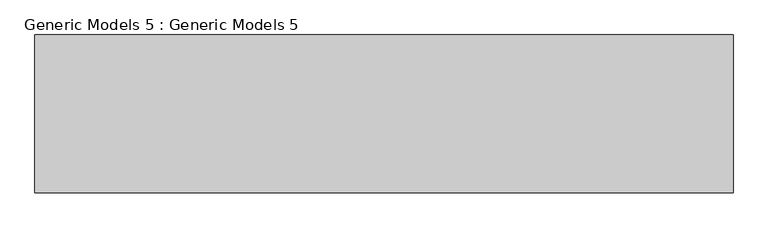
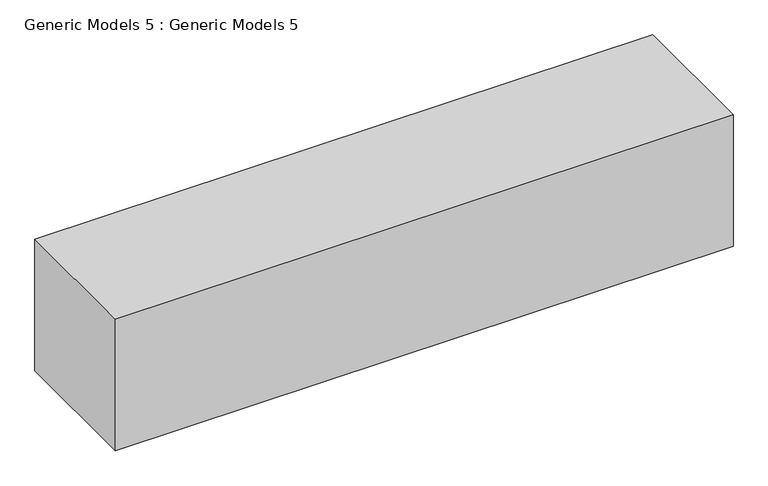
"""IFC4 building model written with IfcOpenShell, lengths in millimetres: proxy geometry, Generic Models 5 : Generic Models 5."""

from ifc_helpers import new_model, si_unit, frame, origin, place, context, project, spatial, polyline, outline, extrude, source, transform, mapped, element, save


def generic_models_5_generic_models_5_ea9a58cb(model_context):
    return source(origin(), model_context, "Body", "SweptSolid", [
        extrude(outline(polyline([(5025.7248685, -14083.1167162), (5025.7248685, -14845.1167162), (1652.8739931, -14845.1167162), (1652.8739931, -14083.1167162), (5025.7248685, -14083.1167162)])), frame((0.0, 0.0, 5799.1653852), z_axis=(0.0, 0.0, 1.0), x_axis=(1.0, 0.0, 0.0)), (0.0, 0.0, 1.0), 757.3100336),
    ])


if __name__ == "__main__":
    model = new_model("IFC4")
    model_context = context("Model", 3, world=origin())
    ifc_project = project(units=[si_unit("LENGTHUNIT", "METRE", prefix="MILLI")], contexts=[model_context])
    site = spatial("IfcSite", under=ifc_project)
    building = spatial("IfcBuilding", under=site)
    placement = place(None, origin())
    generic_models_5_generic_models_5_shape = generic_models_5_generic_models_5_ea9a58cb(model_context)
    element("IfcBuildingElementProxy", 1, Name="Generic Models 5 : Generic Models 5", ObjectType="Generic Models 5 : Generic Models 5", at=placement, inside=building, context=model_context, shape_type="MappedRepresentation", body=[
        mapped(generic_models_5_generic_models_5_shape, transform((0.0, 0.0, 0.0), x_axis=(1.0, 0.0, 0.0), y_axis=(0.0, 1.0, 0.0), z_axis=(0.0, 0.0, 1.0))),
    ])
    save(model, "model.ifc")
